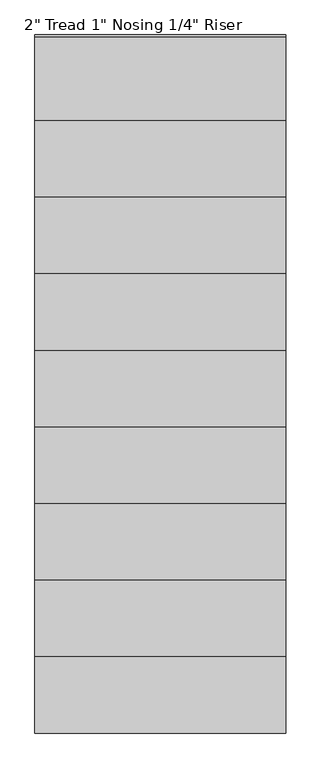
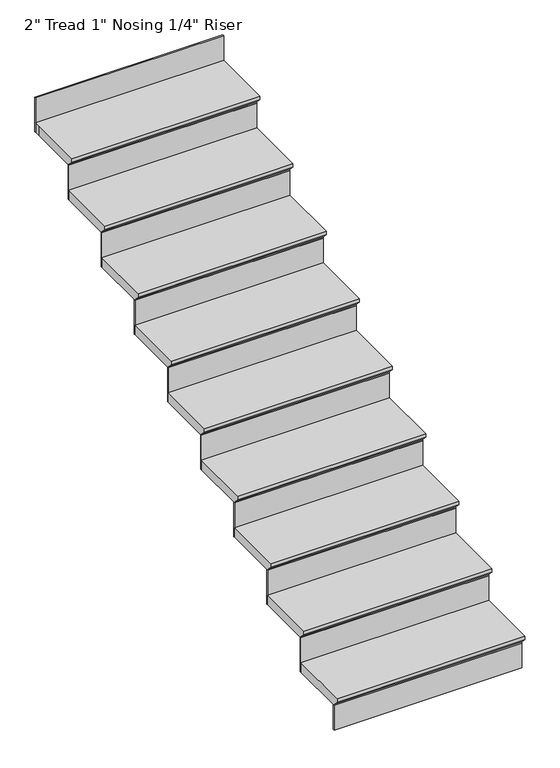
"""IFC4 building model written with IfcOpenShell, lengths in millimetres: stair flight geometry."""

from ifc_helpers import new_model, si_unit, origin, place, context, project, spatial, faceted_brep, source, transform, mapped, element, save


def stair_flight_508a9823(model_context):
    return source(origin(), model_context, "Body", "Brep", [
        faceted_brep([(8378.8260838, -1689.0339187, 3968.75), (8378.8260838, -1689.0339187, 3987.8), (7464.4260838, -1689.0339187, 3987.8), (7464.4260838, -1689.0339187, 3968.75), (8378.8260838, -1663.6339187, 3943.35), (7464.4260838, -1663.6339187, 3943.35), (8378.8260838, -1384.2339187, 3987.8), (7464.4260838, -1384.2339187, 3987.8), (7464.4260838, -1663.6339187, 3937.0), (7464.4260838, -1384.2339187, 3937.0), (8378.8260838, -1384.2339187, 3937.0), (8378.8260838, -1663.6339187, 3937.0)], [[[0, 1, 2, 3]], [[4, 0, 3, 5]], [[2, 1, 6, 7]], [[8, 9, 10, 11]], [[2, 7, 9, 8, 5, 3]], [[8, 11, 4, 5]], [[6, 1, 0, 4, 11, 10]], [[7, 6, 10, 9]]]),
        faceted_brep([(8378.8260838, -1663.6339187, 3937.0), (8378.8260838, -1663.6339187, 3810.0), (8378.8260838, -1657.2839187, 3810.0), (8378.8260838, -1657.2839187, 3937.0), (7464.4260838, -1663.6339187, 3937.0), (7464.4260838, -1657.2839187, 3937.0), (7464.4260838, -1657.2839187, 3810.0), (7464.4260838, -1663.6339187, 3810.0)], [[[0, 1, 2, 3]], [[4, 5, 6, 7]], [[1, 0, 4, 7]], [[2, 1, 7, 6]], [[3, 2, 6, 5]], [[0, 3, 5, 4]]]),
        faceted_brep([(8378.8260838, -1384.2339187, 4114.8), (8378.8260838, -1384.2339187, 3937.0), (8378.8260838, -1377.8839187, 3937.0), (8378.8260838, -1377.8839187, 4114.8), (7464.4260838, -1384.2339187, 4114.8), (7464.4260838, -1377.8839187, 4114.8), (7464.4260838, -1377.8839187, 3937.0), (7464.4260838, -1384.2339187, 3937.0)], [[[0, 1, 2, 3]], [[4, 5, 6, 7]], [[1, 0, 4, 7]], [[2, 1, 7, 6]], [[3, 2, 6, 5]], [[0, 3, 5, 4]]]),
        faceted_brep([(7464.4260838, -1409.6339187, 4165.6), (8378.8260838, -1409.6339187, 4165.6), (8378.8260838, -1104.8339187, 4165.6), (7464.4260838, -1104.8339187, 4165.6), (7464.4260838, -1384.2339187, 4114.8), (7464.4260838, -1104.8339187, 4114.8), (8378.8260838, -1104.8339187, 4114.8), (8378.8260838, -1384.2339187, 4114.8), (7464.4260838, -1384.2339187, 4121.15), (7464.4260838, -1409.6339187, 4146.55), (8378.8260838, -1384.2339187, 4121.15), (8378.8260838, -1409.6339187, 4146.55)], [[[0, 1, 2, 3]], [[4, 5, 6, 7]], [[0, 3, 5, 4, 8, 9]], [[4, 7, 10, 8]], [[2, 1, 11, 10, 7, 6]], [[3, 2, 6, 5]], [[11, 1, 0, 9]], [[10, 11, 9, 8]]]),
        faceted_brep([(8378.8260838, -1104.8339187, 4292.6), (8378.8260838, -1104.8339187, 4114.8), (8378.8260838, -1098.4839187, 4114.8), (8378.8260838, -1098.4839187, 4292.6), (7464.4260838, -1104.8339187, 4292.6), (7464.4260838, -1098.4839187, 4292.6), (7464.4260838, -1098.4839187, 4114.8), (7464.4260838, -1104.8339187, 4114.8)], [[[0, 1, 2, 3]], [[4, 5, 6, 7]], [[1, 0, 4, 7]], [[2, 1, 7, 6]], [[3, 2, 6, 5]], [[0, 3, 5, 4]]]),
        faceted_brep([(7464.4260838, -1130.2339187, 4343.4), (8378.8260838, -1130.2339187, 4343.4), (8378.8260838, -825.4339187, 4343.4), (7464.4260838, -825.4339187, 4343.4), (7464.4260838, -1104.8339187, 4292.6), (7464.4260838, -825.4339187, 4292.6), (8378.8260838, -825.4339187, 4292.6), (8378.8260838, -1104.8339187, 4292.6), (7464.4260838, -1104.8339187, 4298.95), (7464.4260838, -1130.2339187, 4324.35), (8378.8260838, -1104.8339187, 4298.95), (8378.8260838, -1130.2339187, 4324.35)], [[[0, 1, 2, 3]], [[4, 5, 6, 7]], [[0, 3, 5, 4, 8, 9]], [[4, 7, 10, 8]], [[2, 1, 11, 10, 7, 6]], [[3, 2, 6, 5]], [[11, 1, 0, 9]], [[10, 11, 9, 8]]]),
        faceted_brep([(8378.8260838, -825.4339187, 4470.4), (8378.8260838, -825.4339187, 4292.6), (8378.8260838, -819.0839187, 4292.6), (8378.8260838, -819.0839187, 4470.4), (7464.4260838, -825.4339187, 4470.4), (7464.4260838, -819.0839187, 4470.4), (7464.4260838, -819.0839187, 4292.6), (7464.4260838, -825.4339187, 4292.6)], [[[0, 1, 2, 3]], [[4, 5, 6, 7]], [[1, 0, 4, 7]], [[2, 1, 7, 6]], [[3, 2, 6, 5]], [[0, 3, 5, 4]]]),
        faceted_brep([(7464.4260838, -850.8339187, 4521.2), (8378.8260838, -850.8339187, 4521.2), (8378.8260838, -546.0339187, 4521.2), (7464.4260838, -546.0339187, 4521.2), (7464.4260838, -825.4339187, 4470.4), (7464.4260838, -546.0339187, 4470.4), (8378.8260838, -546.0339187, 4470.4), (8378.8260838, -825.4339187, 4470.4), (7464.4260838, -825.4339187, 4476.75), (7464.4260838, -850.8339187, 4502.15), (8378.8260838, -825.4339187, 4476.75), (8378.8260838, -850.8339187, 4502.15)], [[[0, 1, 2, 3]], [[4, 5, 6, 7]], [[0, 3, 5, 4, 8, 9]], [[4, 7, 10, 8]], [[2, 1, 11, 10, 7, 6]], [[3, 2, 6, 5]], [[11, 1, 0, 9]], [[10, 11, 9, 8]]]),
        faceted_brep([(8378.8260838, -546.0339187, 4648.2), (8378.8260838, -546.0339187, 4470.4), (8378.8260838, -539.6839187, 4470.4), (8378.8260838, -539.6839187, 4648.2), (7464.4260838, -546.0339187, 4648.2), (7464.4260838, -539.6839187, 4648.2), (7464.4260838, -539.6839187, 4470.4), (7464.4260838, -546.0339187, 4470.4)], [[[0, 1, 2, 3]], [[4, 5, 6, 7]], [[1, 0, 4, 7]], [[2, 1, 7, 6]], [[3, 2, 6, 5]], [[0, 3, 5, 4]]]),
        faceted_brep([(7464.4260838, -571.4339187, 4699.0), (8378.8260838, -571.4339187, 4699.0), (8378.8260838, -266.6339187, 4699.0), (7464.4260838, -266.6339187, 4699.0), (7464.4260838, -546.0339187, 4648.2), (7464.4260838, -266.6339187, 4648.2), (8378.8260838, -266.6339187, 4648.2), (8378.8260838, -546.0339187, 4648.2), (7464.4260838, -546.0339187, 4654.55), (7464.4260838, -571.4339187, 4679.95), (8378.8260838, -546.0339187, 4654.55), (8378.8260838, -571.4339187, 4679.95)], [[[0, 1, 2, 3]], [[4, 5, 6, 7]], [[0, 3, 5, 4, 8, 9]], [[4, 7, 10, 8]], [[2, 1, 11, 10, 7, 6]], [[3, 2, 6, 5]], [[11, 1, 0, 9]], [[10, 11, 9, 8]]]),
        faceted_brep([(8378.8260838, -266.6339187, 4826.0), (8378.8260838, -266.6339187, 4648.2), (8378.8260838, -260.2839187, 4648.2), (8378.8260838, -260.2839187, 4826.0), (7464.4260838, -266.6339187, 4826.0), (7464.4260838, -260.2839187, 4826.0), (7464.4260838, -260.2839187, 4648.2), (7464.4260838, -266.6339187, 4648.2)], [[[0, 1, 2, 3]], [[4, 5, 6, 7]], [[1, 0, 4, 7]], [[2, 1, 7, 6]], [[3, 2, 6, 5]], [[0, 3, 5, 4]]]),
        faceted_brep([(7464.4260838, -292.0339187, 4876.8), (8378.8260838, -292.0339187, 4876.8), (8378.8260838, 12.7660813, 4876.8), (7464.4260838, 12.7660813, 4876.8), (7464.4260838, -266.6339187, 4826.0), (7464.4260838, 12.7660813, 4826.0), (8378.8260838, 12.7660813, 4826.0), (8378.8260838, -266.6339187, 4826.0), (7464.4260838, -266.6339187, 4832.35), (7464.4260838, -292.0339187, 4857.75), (8378.8260838, -266.6339187, 4832.35), (8378.8260838, -292.0339187, 4857.75)], [[[0, 1, 2, 3]], [[4, 5, 6, 7]], [[0, 3, 5, 4, 8, 9]], [[4, 7, 10, 8]], [[2, 1, 11, 10, 7, 6]], [[3, 2, 6, 5]], [[11, 1, 0, 9]], [[10, 11, 9, 8]]]),
        faceted_brep([(8378.8260838, 12.7660813, 5003.8), (8378.8260838, 12.7660813, 4826.0), (8378.8260838, 19.1160813, 4826.0), (8378.8260838, 19.1160813, 5003.8), (7464.4260838, 12.7660813, 5003.8), (7464.4260838, 19.1160813, 5003.8), (7464.4260838, 19.1160813, 4826.0), (7464.4260838, 12.7660813, 4826.0)], [[[0, 1, 2, 3]], [[4, 5, 6, 7]], [[1, 0, 4, 7]], [[2, 1, 7, 6]], [[3, 2, 6, 5]], [[0, 3, 5, 4]]]),
        faceted_brep([(7464.4260838, -12.6339187, 5054.6), (8378.8260838, -12.6339187, 5054.6), (8378.8260838, 292.1660813, 5054.6), (7464.4260838, 292.1660813, 5054.6), (7464.4260838, 12.7660813, 5003.8), (7464.4260838, 292.1660813, 5003.8), (8378.8260838, 292.1660813, 5003.8), (8378.8260838, 12.7660813, 5003.8), (7464.4260838, 12.7660813, 5010.15), (7464.4260838, -12.6339187, 5035.55), (8378.8260838, 12.7660813, 5010.15), (8378.8260838, -12.6339187, 5035.55)], [[[0, 1, 2, 3]], [[4, 5, 6, 7]], [[0, 3, 5, 4, 8, 9]], [[4, 7, 10, 8]], [[2, 1, 11, 10, 7, 6]], [[3, 2, 6, 5]], [[11, 1, 0, 9]], [[10, 11, 9, 8]]]),
        faceted_brep([(8378.8260838, 292.1660813, 5181.6), (8378.8260838, 292.1660813, 5003.8), (8378.8260838, 298.5160813, 5003.8), (8378.8260838, 298.5160813, 5181.6), (7464.4260838, 292.1660813, 5181.6), (7464.4260838, 298.5160813, 5181.6), (7464.4260838, 298.5160813, 5003.8), (7464.4260838, 292.1660813, 5003.8)], [[[0, 1, 2, 3]], [[4, 5, 6, 7]], [[1, 0, 4, 7]], [[2, 1, 7, 6]], [[3, 2, 6, 5]], [[0, 3, 5, 4]]]),
        faceted_brep([(7464.4260838, 266.7660813, 5232.4), (8378.8260838, 266.7660813, 5232.4), (8378.8260838, 571.5660813, 5232.4), (7464.4260838, 571.5660813, 5232.4), (7464.4260838, 292.1660813, 5181.6), (7464.4260838, 571.5660813, 5181.6), (8378.8260838, 571.5660813, 5181.6), (8378.8260838, 292.1660813, 5181.6), (7464.4260838, 292.1660813, 5187.95), (7464.4260838, 266.7660813, 5213.35), (8378.8260838, 292.1660813, 5187.95), (8378.8260838, 266.7660813, 5213.35)], [[[0, 1, 2, 3]], [[4, 5, 6, 7]], [[0, 3, 5, 4, 8, 9]], [[4, 7, 10, 8]], [[2, 1, 11, 10, 7, 6]], [[3, 2, 6, 5]], [[11, 1, 0, 9]], [[10, 11, 9, 8]]]),
        faceted_brep([(8378.8260838, 850.9660813, 5537.2), (8378.8260838, 850.9660813, 5359.4), (8378.8260838, 857.3160813, 5359.4), (8378.8260838, 857.3160813, 5537.2), (7464.4260838, 850.9660813, 5537.2), (7464.4260838, 857.3160813, 5537.2), (7464.4260838, 857.3160813, 5359.4), (7464.4260838, 850.9660813, 5359.4)], [[[0, 1, 2, 3]], [[4, 5, 6, 7]], [[1, 0, 4, 7]], [[2, 1, 7, 6]], [[3, 2, 6, 5]], [[0, 3, 5, 4]]]),
        faceted_brep([(8378.8260838, 571.5660813, 5359.4), (8378.8260838, 571.5660813, 5181.6), (8378.8260838, 577.9160813, 5181.6), (8378.8260838, 577.9160813, 5359.4), (7464.4260838, 571.5660813, 5359.4), (7464.4260838, 577.9160813, 5359.4), (7464.4260838, 577.9160813, 5181.6), (7464.4260838, 571.5660813, 5181.6)], [[[0, 1, 2, 3]], [[4, 5, 6, 7]], [[1, 0, 4, 7]], [[2, 1, 7, 6]], [[3, 2, 6, 5]], [[0, 3, 5, 4]]]),
        faceted_brep([(7464.4260838, 850.9660813, 5410.2), (7464.4260838, 825.5660813, 5410.2), (7464.4260838, 546.1660813, 5410.2), (8378.8260838, 546.1660813, 5410.2), (8378.8260838, 850.9660813, 5410.2), (7464.4260838, 825.5660813, 5359.4), (7464.4260838, 850.9660813, 5359.4), (8378.8260838, 850.9660813, 5359.4), (8378.8260838, 571.5660813, 5359.4), (7464.4260838, 571.5660813, 5359.4), (7464.4260838, 571.5660813, 5365.75), (7464.4260838, 546.1660813, 5391.15), (8378.8260838, 571.5660813, 5365.75), (8378.8260838, 546.1660813, 5391.15)], [[[0, 1, 2, 3, 4]], [[5, 6, 7, 8, 9]], [[1, 0, 6, 5]], [[2, 1, 5, 9, 10, 11]], [[9, 8, 12, 10]], [[4, 3, 13, 12, 8, 7]], [[0, 4, 7, 6]], [[13, 3, 2, 11]], [[12, 13, 11, 10]]]),
    ])


if __name__ == "__main__":
    model = new_model("IFC4")
    model_context = context("Model", 3, world=origin())
    ifc_project = project(units=[si_unit("LENGTHUNIT", "METRE", prefix="MILLI")], contexts=[model_context])
    site = spatial("IfcSite", under=ifc_project)
    building = spatial("IfcBuilding", under=site)
    placement = place(None, origin())
    stair_flight_shape = stair_flight_508a9823(model_context)
    element("IfcStairFlight", 1, ObjectType="2\" Tread 1\" Nosing 1/4\" Riser", at=placement, inside=building, context=model_context, shape_type="MappedRepresentation", body=[
        mapped(stair_flight_shape, transform((0.0, 0.0, 0.0), x_axis=(1.0, 0.0, 0.0), y_axis=(0.0, 1.0, 0.0), z_axis=(0.0, 0.0, 1.0))),
    ])
    save(model, "model.ifc")
